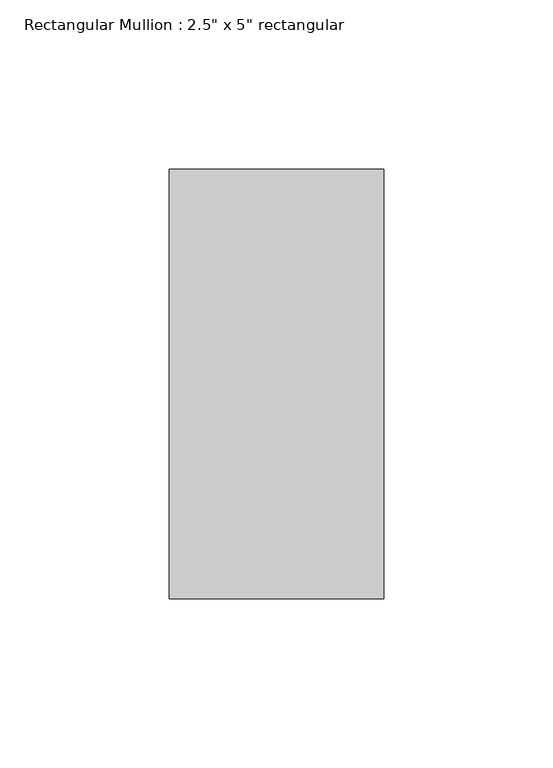
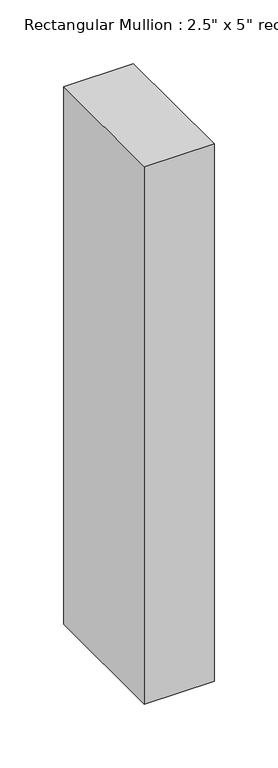
"""IFC4 building model written with IfcOpenShell, lengths in millimetres: member geometry."""

from ifc_helpers import new_model, si_unit, frame, origin, place, context, project, spatial, polyline, outline, extrude, source, transform, mapped, element, save


def member_b3098cb3(model_context):
    return source(origin(), model_context, "Body", "SweptSolid", [
        extrude(outline(polyline([(31.75, 63.5), (31.75, -63.5), (-31.75, -63.5), (-31.75, 63.5), (31.75, 63.5)])), frame((0.0, 0.0, -516.4666667), z_axis=(0.0, 0.0, 1.0), x_axis=(1.0, 0.0, 0.0)), (0.0, 0.0, 1.0), 516.4666667),
    ])


if __name__ == "__main__":
    model = new_model("IFC4")
    model_context = context("Model", 3, world=origin())
    ifc_project = project(units=[si_unit("LENGTHUNIT", "METRE", prefix="MILLI")], contexts=[model_context])
    site = spatial("IfcSite", under=ifc_project)
    building = spatial("IfcBuilding", under=site)
    placement = place(None, origin())
    member_shape = member_b3098cb3(model_context)
    element("IfcMember", 1, ObjectType="Rectangular Mullion : 2.5\" x 5\" rectangular", at=placement, inside=building, context=model_context, shape_type="MappedRepresentation", body=[
        mapped(member_shape, transform((0.0, 0.0, 0.0), x_axis=(1.0, 0.0, 0.0), y_axis=(0.0, 1.0, 0.0), z_axis=(0.0, 0.0, 1.0))),
    ])
    save(model, "model.ifc")

# Revit data of these elements
# Type "Rectangular Mullion : 2.5\" x 5\" rectangular"
#   built-in parameter 1007304 = 0.416667 (stored number, unit not read)
#   built-in parameter 1007301 = 0.104167 (stored number, unit not read)
#   built-in parameter 1007300 = 0.104167 (stored number, unit not read)
